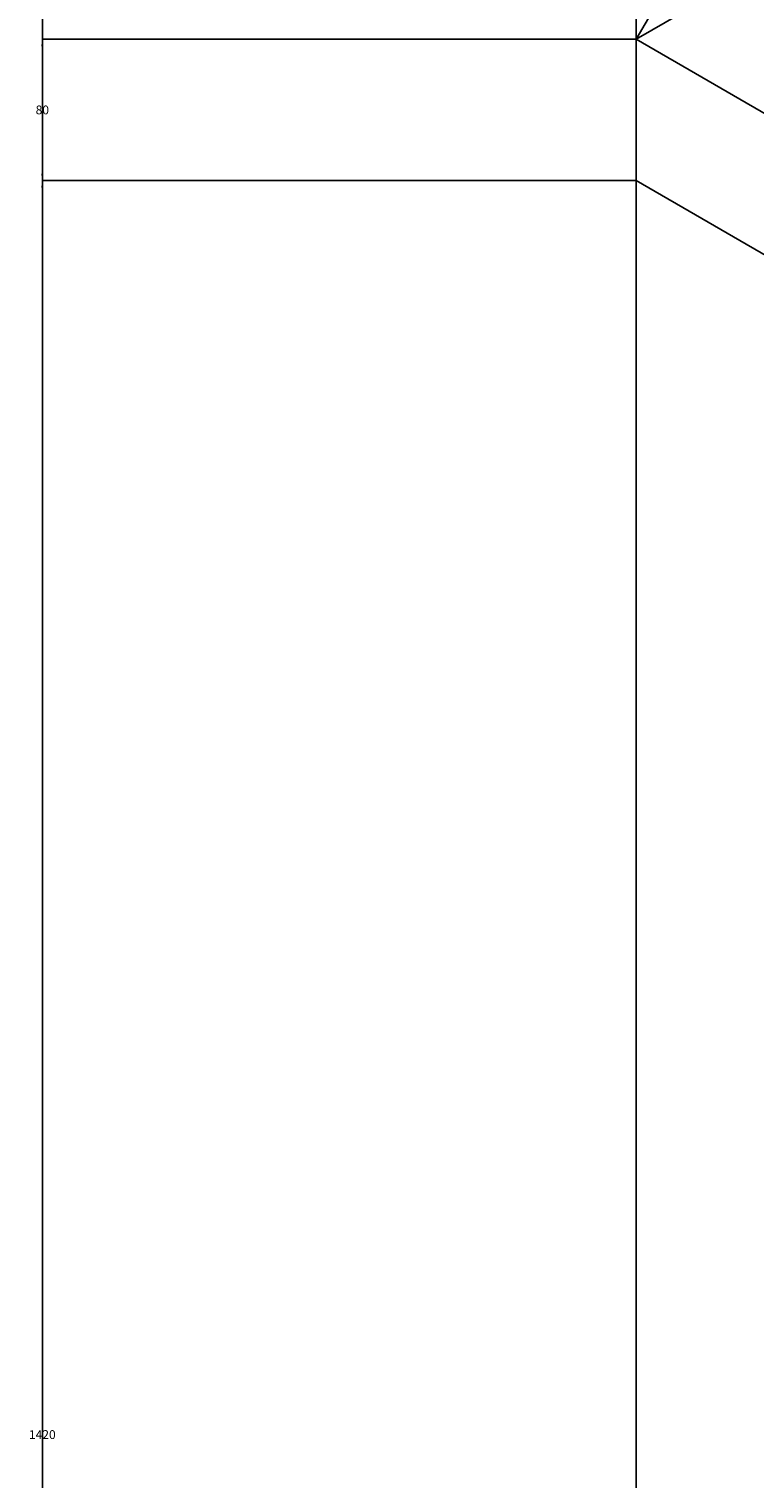
# Model space of a CAD drawing. Units: metres. Extents: x -2391 to 4922, y -635 to 4845.
# Tile 14 of 37: x -2391 to -1981, y 2190 to 3011. Entities that reach past the tile are written whole.
import ezdxf

# ---------------------------------------------------------------- set-up
doc = ezdxf.new("R2010")
doc.units = ezdxf.units.M
doc.header["$MEASUREMENT"] = 0
doc.layers.add('A-ANNO-DIMS', color=2, linetype='Continuous', lineweight=18)
doc.layers.add('A-FLOR-FIXT', color=3, linetype='Continuous', lineweight=25)
doc.styles.get("Standard").update_dxf_attribs({"font": 'arial.ttf'})
doc.dimstyles.get("Standard").update_dxf_attribs({"dimtxt": 5, "dimasz": 4, "dimexe": 0.18, "dimexo": 0.0625, "dimgap": 0.09, "dimtad": 0, "dimtih": 1, "dimtoh": 1, "dimdec": 0, "dimzin": 0, "dimdsep": 46, "dimtxsty": 'Standard', "dimcen": 0.09, "dimadec": 0, "dimazin": 0, "dimtfac": 1, "dimtdec": 0, "dimtofl": 0, "dimtmove": 0, "dimatfit": 3, "dimfxl": 1, "dimtolj": 1, "dimtzin": 0, "dimarcsym": 0})

# ---------------------------------------------------------------- blocks, each defined once
blk = doc.blocks.new('*D8')
at = {"layer": 'A-ANNO-DIMS', "color": 0, "lineweight": -2, "transparency": 16777216}
for p, q in [((-2047.33, 3005.21), (-2047.33, -631.4)), ((4577.76, 2350.21), (4577.76, -631.4)), ((-2043.33, -631.22), (1257.62, -631.22)), ((4573.76, -631.22), (1272.8, -631.22))]:
    blk.add_line(p, q, dxfattribs=at)
at = {"layer": 'A-ANNO-DIMS', "color": 0, "transparency": 16777216}
for points in [[(-2043.33, -630.56), (-2043.33, -631.89), (-2047.33, -631.22)], [(4573.76, -630.56), (4573.76, -631.89), (4577.76, -631.22)]]:
    blk.add_solid(points, dxfattribs=at)
at = {"layer": 'Defpoints', "color": 0, "transparency": 16777216}
for p in [(-2047.33, 3005.28), (4577.76, 2350.28), (4577.76, -631.22)]:
    blk.add_point(p, dxfattribs=at)
at = {"layer": 'A-ANNO-DIMS', "color": 0, "transparency": 16777216, "insert": (1265.21, -631.22), "char_height": 5, "attachment_point": 5}
blk.add_mtext('\\A1;6625', dxfattribs=at)
blk = doc.blocks.new('*D9')
at = {"layer": 'A-ANNO-DIMS', "color": 0, "lineweight": -2, "transparency": 16777216}
for p, q in [((-2047.33, 3005.34), (-2047.33, 4841.96)), ((-2043.33, 4841.78), (-755.9, 4841.78)), ((546.74, 4841.78), (-740.69, 4841.78)), ((550.74, 4505.34), (550.74, 4841.96))]:
    blk.add_line(p, q, dxfattribs=at)
at = {"layer": 'A-ANNO-DIMS', "color": 0, "transparency": 16777216}
for points in [[(-2043.33, 4842.44), (-2043.33, 4841.11), (-2047.33, 4841.78)], [(546.74, 4842.44), (546.74, 4841.11), (550.74, 4841.78)]]:
    blk.add_solid(points, dxfattribs=at)
at = {"layer": 'Defpoints', "color": 0, "transparency": 16777216}
for p in [(550.74, 4841.78), (550.74, 4505.28), (-2047.33, 3005.28)]:
    blk.add_point(p, dxfattribs=at)
at = {"layer": 'A-ANNO-DIMS', "color": 0, "transparency": 16777216, "insert": (-748.3, 4841.78), "char_height": 5, "attachment_point": 5}
blk.add_mtext('\\A1;2598', dxfattribs=at)
blk = doc.blocks.new('*D10')
at = {"layer": 'A-ANNO-DIMS', "color": 0, "lineweight": -2, "transparency": 16777216}
for p, q in [((550.68, 4505.28), (-2384.01, 4505.28)), ((-2383.83, 4501.28), (-2383.83, 2107.92)), ((-2383.83, -290.72), (-2383.83, 2102.63)), ((-488.55, -294.72), (-2384.01, -294.72))]:
    blk.add_line(p, q, dxfattribs=at)
at = {"layer": 'A-ANNO-DIMS', "color": 0, "transparency": 16777216}
for points in [[(-2384.5, 4501.28), (-2383.17, 4501.28), (-2383.83, 4505.28)], [(-2384.5, -290.72), (-2383.17, -290.72), (-2383.83, -294.72)]]:
    blk.add_solid(points, dxfattribs=at)
at = {"layer": 'Defpoints', "color": 0, "transparency": 16777216}
for p in [(-2383.83, 4505.28), (550.74, 4505.28), (-488.49, -294.72)]:
    blk.add_point(p, dxfattribs=at)
at = {"layer": 'A-ANNO-DIMS', "color": 0, "transparency": 16777216, "insert": (-2383.83, 2105.28), "char_height": 5, "attachment_point": 5}
blk.add_mtext('\\A1;4800', dxfattribs=at)
blk = doc.blocks.new('*D41')
at = {"layer": 'A-ANNO-DIMS', "color": 0, "lineweight": -2, "transparency": 16777216}
for p, q in [((-2047.3, 3005.33), (-1878.99, 3296.85)), ((-1875.62, 3294.69), (-1104.24, 2849.34)), ((-323.7, 2398.69), (-1095.08, 2844.05)), ((-488.46, 2105.33), (-320.15, 2396.85))]:
    blk.add_line(p, q, dxfattribs=at)
at = {"layer": 'A-ANNO-DIMS', "color": 0, "transparency": 16777216}
for points in [[(-1875.29, 3295.27), (-1875.95, 3294.12), (-1879.08, 3296.69)], [(-323.37, 2399.27), (-324.04, 2398.12), (-320.24, 2396.69)]]:
    blk.add_solid(points, dxfattribs=at)
at = {"layer": 'Defpoints', "color": 0, "transparency": 16777216}
for p in [(-2047.33, 3005.28), (-320.24, 2396.69), (-488.49, 2105.28)]:
    blk.add_point(p, dxfattribs=at)
at = {"layer": 'A-ANNO-DIMS', "color": 0, "transparency": 16777216, "insert": (-1099.66, 2846.69), "char_height": 5, "attachment_point": 5}
blk.add_mtext('\\A1;1800', dxfattribs=at)
blk = doc.blocks.new('*D43')
at = {"layer": 'A-ANNO-DIMS', "color": 0, "lineweight": -2, "transparency": 16777216}
for p, q in [((-2047.4, 2925.28), (-2384.01, 2925.28)), ((-2383.83, 2921.28), (-2383.83, 2217.92)), ((-2383.83, 1509.28), (-2383.83, 2212.63)), ((-2047.4, 1505.28), (-2384.01, 1505.28))]:
    blk.add_line(p, q, dxfattribs=at)
at = {"layer": 'A-ANNO-DIMS', "color": 0, "transparency": 16777216}
for points in [[(-2384.5, 2921.28), (-2383.17, 2921.28), (-2383.83, 2925.28)], [(-2384.5, 1509.28), (-2383.17, 1509.28), (-2383.83, 1505.28)]]:
    blk.add_solid(points, dxfattribs=at)
at = {"layer": 'Defpoints', "color": 0, "transparency": 16777216}
for p in [(-2047.33, 2925.28), (-2383.83, 1505.28), (-2047.33, 1505.28)]:
    blk.add_point(p, dxfattribs=at)
at = {"layer": 'A-ANNO-DIMS', "color": 0, "transparency": 16777216, "insert": (-2383.83, 2215.28), "char_height": 5, "attachment_point": 5}
blk.add_mtext('\\A1;1420', dxfattribs=at)
blk = doc.blocks.new('*D45')
at = {"layer": 'A-ANNO-DIMS', "color": 0, "lineweight": -2, "transparency": 16777216}
for p, q in [((-2047.4, 3005.28), (-2384.01, 3005.28)), ((-2383.83, 3001.28), (-2383.83, 2967.92)), ((-2383.83, 2929.28), (-2383.83, 2962.63)), ((-2047.4, 2925.28), (-2384.01, 2925.28))]:
    blk.add_line(p, q, dxfattribs=at)
at = {"layer": 'A-ANNO-DIMS', "color": 0, "transparency": 16777216}
for points in [[(-2384.5, 3001.28), (-2383.17, 3001.28), (-2383.83, 3005.28)], [(-2384.5, 2929.28), (-2383.17, 2929.28), (-2383.83, 2925.28)]]:
    blk.add_solid(points, dxfattribs=at)
at = {"layer": 'Defpoints', "color": 0, "transparency": 16777216}
for p in [(-2047.33, 3005.28), (-2383.83, 2925.28), (-2047.33, 2925.28)]:
    blk.add_point(p, dxfattribs=at)
at = {"layer": 'A-ANNO-DIMS', "color": 0, "transparency": 16777216, "insert": (-2383.83, 2965.28), "char_height": 5, "attachment_point": 5}
blk.add_mtext('\\A1;80', dxfattribs=at)

msp = doc.modelspace()

# ---------------------------------------------------------------- linework, layer by layer
at = {"layer": 'A-FLOR-FIXT'}
for p, q in [((-2047.3343, 3005.2763), (-1008.1038, 3605.2763)), ((-2047.3343, 1505.2763), (-2047.3343, 3005.2763)), ((-2047.3343, 3005.2763), (-488.4886, 2105.2763)), ((-1240.7842, 2459.6143), (-2047.3343, 2925.2763))]:
    msp.add_line(p, q, dxfattribs=at)

# ---------------------------------------------------------------- dimensions: what is measured, and where the dimension line sits
at = {"layer": 'A-ANNO-DIMS'}
for base, p2, picture, middle in [((550.7419, 4841.7763), (550.7419, 4505.2763), '*D9', (-748.2962, 4841.7763)), ((4577.76, -631.2237), (4577.76, 2350.2763), '*D8', (1265.2128, -631.2237))]:
    dim = msp.add_linear_dim(base=base, p1=(-2047.3343, 3005.2763), p2=p2, dimstyle='Standard', override={"dimdec": 0, "dimlfac": 1, "dimrnd": 0, "dimzin": 0, "dimdsep": 46, "dimlunit": 2}, dxfattribs=at)
    dim.commit()
    dim.dimension.update_dxf_attribs({"geometry": picture, "text_midpoint": middle})
for base, p1, p2, angle, picture, middle in [((-2383.8343, 4505.2763), (-488.4886, -294.7237), (550.7419, 4505.2763), 90, '*D10', (-2383.8343, 2105.2763)), ((-320.2386, 2396.6938), (-2047.3343, 3005.2763), (-488.4886, 2105.2763), 330, '*D41', (-1099.6615, 2846.6938)), ((-2383.8343, 2925.2763), (-2047.3343, 3005.2763), (-2047.3343, 2925.2763), 90, '*D45', (-2383.8343, 2965.2763)), ((-2383.8343, 1505.2763), (-2047.3343, 2925.2763), (-2047.3343, 1505.2763), 90, '*D43', (-2383.8343, 2215.2763))]:
    dim = msp.add_linear_dim(base=base, p1=p1, p2=p2, angle=angle, dimstyle='Standard', override={"dimdec": 0, "dimlfac": 1, "dimrnd": 0, "dimzin": 0, "dimdsep": 46, "dimlunit": 2}, dxfattribs=at)
    dim.commit()
    dim.dimension.update_dxf_attribs({"geometry": picture, "text_midpoint": middle})

doc.saveas('drawing.dxf')
